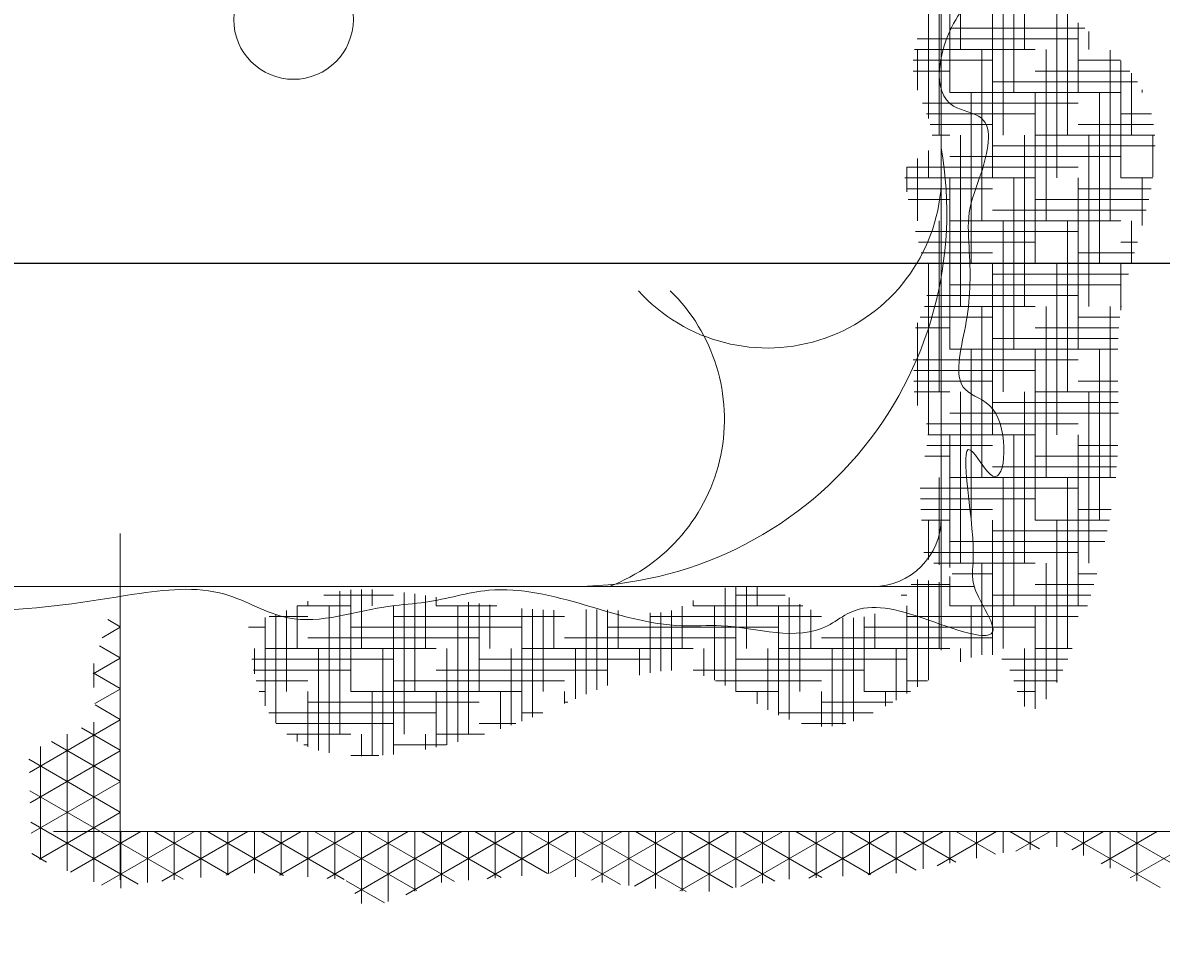
# Model space of a CAD drawing. Units: inches. Extents: x 3731 to 4318, y 1310 to 2388.
# Tile 52 of 57: x 4157 to 4212, y 2229 to 2274. Entities that reach past the tile are written whole.
import ezdxf

# ---------------------------------------------------------------- set-up
doc = ezdxf.new("R2010")
doc.units = ezdxf.units.IN
doc.layers.add('A-ANNO-DIMS', color=2, linetype='Continuous', lineweight=18)
doc.layers.add('A-FURN', color=8, linetype='Continuous', lineweight=13)
doc.styles.get("Standard").update_dxf_attribs({"font": 'arial.ttf'})
doc.dimstyles.get("Standard").update_dxf_attribs({"dimtxt": 0.18, "dimasz": 0.18, "dimexe": 0.18, "dimexo": 0.0625, "dimgap": 0.09, "dimtad": 0, "dimtih": 1, "dimtoh": 1, "dimdec": 4, "dimzin": 0, "dimdsep": 46, "dimtxsty": 'Standard', "dimcen": 0.09, "dimadec": 0, "dimazin": 0, "dimtfac": 1, "dimtdec": 4, "dimtofl": 0, "dimtmove": 0, "dimatfit": 3, "dimfxl": 1, "dimtolj": 1, "dimtzin": 0, "dimarcsym": 0})

# ---------------------------------------------------------------- blocks, each defined once
blk = doc.blocks.new('A$C200C7901')
for p, q in [((2, 0.2957), (2, 1.2957)), ((2.0224, 0.9977), (2.0224, 1.1977)), ((2.0224, 0.9977), (2.0224, 1.1977)), ((1.9974, 0.5977), (1.9974, 0.7977)), ((1.9974, 0.5977), (1.9974, 0.7977)), ((2.0724, 0.5977), (2.0724, 0.7977)), ((2.0724, 0.5977), (2.0724, 0.7977)), ((2.1474, 0.5977), (2.1474, 0.7977)), ((2.1474, 0.5977), (2.1474, 0.7977)), ((1.9849, 0.5477), (1.9849, 0.7477)), ((1.9849, 0.5477), (1.9849, 0.7477)), ((2.0599, 0.5477), (2.0599, 0.7477)), ((2.0599, 0.5477), (2.0599, 0.7477)), ((2.1349, 0.5477), (2.1349, 0.7477)), ((2.1349, 0.5477), (2.1349, 0.7477)), ((1.0407, 0.0275), (1.0407, 0.4323)), ((0.4061, 0.3703), (2.0386, 0.3703)), ((2.4073, 0.0839), (0.9625, 0.0839))]:
    blk.add_line(p, q)
at = {"linetype": 'ByBlock'}
for p, q in [((2.0099, 0.9477), (2.0099, 1.1477)), ((2.0099, 0.9477), (2.0099, 1.1477)), ((2.0849, 0.9477), (2.0849, 1.1477)), ((2.0849, 0.9477), (2.0849, 1.1477)), ((1.9974, 0.8977), (1.9974, 1.0977)), ((1.9974, 0.8977), (1.9974, 1.0977)), ((2.0724, 0.8977), (2.0724, 1.0977)), ((2.0724, 0.8977), (2.0724, 1.0977)), ((2.0974, 0.9977), (2.0974, 1.0909)), ((2.0974, 0.9977), (2.0974, 1.0909)), ((1.9849, 0.9171), (1.9849, 1.0477)), ((1.9849, 0.9171), (1.9849, 1.0477)), ((2.0599, 0.8477), (2.0599, 1.0477)), ((2.0599, 0.8477), (2.0599, 1.0477)), ((2.1349, 0.8477), (2.1349, 1.0477)), ((2.1349, 0.8477), (2.1349, 1.0477)), ((2.1474, 0.8977), (2.1474, 1.0391)), ((2.1474, 0.8977), (2.1474, 1.0391)), ((2.1599, 0.9477), (2.1599, 1.029)), ((2.1599, 0.9477), (2.1599, 1.029)), ((2.0099, 1.0227), (2.1678, 1.0227)), ((2.0099, 1.0227), (2.1678, 1.0227)), ((2.1724, 0.9977), (2.1724, 1.0189)), ((2.1724, 0.9977), (2.1724, 1.0189)), ((1.9718, 1.0102), (2.1599, 1.0102)), ((1.9718, 1.0102), (2.1599, 1.0102)), ((1.9671, 0.9852), (2.0599, 0.9852)), ((1.9671, 0.9852), (2.0599, 0.9852)), ((1.9688, 0.9977), (2.1099, 0.9977)), ((1.9688, 0.9977), (2.1099, 0.9977)), ((1.9724, 0.9504), (1.9724, 0.9977)), ((1.9724, 0.9504), (1.9724, 0.9977)), ((2.0474, 0.7977), (2.0474, 0.9977)), ((2.0474, 0.7977), (2.0474, 0.9977)), ((2.1224, 0.7977), (2.1224, 0.9977)), ((2.1224, 0.7977), (2.1224, 0.9977)), ((2.1599, 0.9852), (2.2095, 0.9852)), ((2.1599, 0.9852), (2.2095, 0.9852)), ((2.1974, 0.7977), (2.1974, 0.9972)), ((2.1974, 0.7977), (2.1974, 0.9972)), ((2.2099, 0.8477), (2.2099, 0.9848)), ((2.2099, 0.8477), (2.2099, 0.9848)), ((1.9672, 0.9727), (2.0099, 0.9727)), ((1.9672, 0.9727), (2.0099, 0.9727)), ((2.1099, 0.9727), (2.2204, 0.9727)), ((2.1099, 0.9727), (2.2204, 0.9727)), ((2.0599, 0.9602), (2.2294, 0.9602)), ((2.0599, 0.9602), (2.2294, 0.9602)), ((2.2224, 0.8977), (2.2224, 0.9702)), ((2.2224, 0.8977), (2.2224, 0.9702)), ((2.0099, 0.9477), (2.2099, 0.9477)), ((2.0099, 0.9477), (2.2099, 0.9477)), ((2.0349, 0.7477), (2.0349, 0.9477)), ((2.0349, 0.7477), (2.0349, 0.9477)), ((2.1099, 0.7477), (2.1099, 0.9477)), ((2.1099, 0.7477), (2.1099, 0.9477)), ((2.1849, 0.7477), (2.1849, 0.9477)), ((2.1849, 0.7477), (2.1849, 0.9477)), ((2.2349, 0.9477), (2.2349, 0.9506)), ((2.2349, 0.9477), (2.2349, 0.9506)), ((1.9781, 0.9352), (2.1599, 0.9352)), ((1.9781, 0.9352), (2.1599, 0.9352)), ((1.9829, 0.9227), (2.1099, 0.9227)), ((1.9829, 0.9227), (2.1099, 0.9227)), ((2.2099, 0.9227), (2.2455, 0.9227)), ((2.2099, 0.9227), (2.2455, 0.9227)), ((1.9871, 0.9102), (2.0599, 0.9102)), ((1.9871, 0.9102), (2.0599, 0.9102)), ((2.1599, 0.9102), (2.2481, 0.9102)), ((2.1599, 0.9102), (2.2481, 0.9102)), ((1.9894, 0.8977), (2.0099, 0.8977)), ((1.9894, 0.8977), (2.0099, 0.8977)), ((2.0224, 0.6977), (2.0224, 0.8977)), ((2.0224, 0.6977), (2.0224, 0.8977)), ((2.0974, 0.6977), (2.0974, 0.8977)), ((2.0974, 0.6977), (2.0974, 0.8977)), ((2.1099, 0.8977), (2.2496, 0.8977)), ((2.1099, 0.8977), (2.2496, 0.8977)), ((2.1724, 0.6977), (2.1724, 0.8977)), ((2.1724, 0.6977), (2.1724, 0.8977)), ((2.2474, 0.8489), (2.2474, 0.8977)), ((2.2474, 0.8489), (2.2474, 0.8977)), ((1.9849, 0.8477), (1.9849, 0.88)), ((1.9849, 0.8477), (1.9849, 0.88)), ((2.0599, 0.8852), (2.2501, 0.8852)), ((2.0599, 0.8852), (2.2501, 0.8852)), ((1.9724, 0.7977), (1.9724, 0.8703)), ((1.9724, 0.7977), (1.9724, 0.8703)), ((2.0099, 0.8727), (2.2099, 0.8727)), ((2.0099, 0.8727), (2.2099, 0.8727)), ((1.9599, 0.8317), (1.9599, 0.8604)), ((1.9599, 0.8317), (1.9599, 0.8604)), ((1.9599, 0.8602), (2.1599, 0.8602)), ((1.9599, 0.8602), (2.1599, 0.8602)), ((1.9574, 0.8477), (2.1099, 0.8477)), ((1.9574, 0.8477), (2.1099, 0.8477)), ((2.0099, 0.6477), (2.0099, 0.8477)), ((2.0099, 0.6477), (2.0099, 0.8477)), ((2.0849, 0.6477), (2.0849, 0.8477)), ((2.0849, 0.6477), (2.0849, 0.8477)), ((2.1599, 0.6477), (2.1599, 0.8477)), ((2.1599, 0.6477), (2.1599, 0.8477)), ((2.2099, 0.8477), (2.2472, 0.8477)), ((2.2099, 0.8477), (2.2472, 0.8477)), ((2.2349, 0.7923), (2.2349, 0.8477)), ((2.2349, 0.7923), (2.2349, 0.8477)), ((1.9593, 0.8352), (2.0599, 0.8352)), ((1.9593, 0.8352), (2.0599, 0.8352)), ((2.1599, 0.8352), (2.2451, 0.8352)), ((2.1599, 0.8352), (2.2451, 0.8352)), ((1.9615, 0.8227), (2.0099, 0.8227)), ((1.9615, 0.8227), (2.0099, 0.8227)), ((2.1099, 0.8227), (2.2425, 0.8227)), ((2.1099, 0.8227), (2.2425, 0.8227)), ((2.0599, 0.8102), (2.2396, 0.8102)), ((2.0599, 0.8102), (2.2396, 0.8102)), ((1.9699, 0.7852), (2.1599, 0.7852)), ((1.9699, 0.7852), (2.1599, 0.7852)), ((2.0099, 0.7977), (2.2099, 0.7977)), ((2.0099, 0.7977), (2.2099, 0.7977)), ((2.2224, 0.7483), (2.2224, 0.7977)), ((2.2224, 0.7483), (2.2224, 0.7977)), ((1.9734, 0.7727), (2.1099, 0.7727)), ((1.9734, 0.7727), (2.1099, 0.7727)), ((2.2099, 0.7727), (2.2294, 0.7727)), ((2.2099, 0.7727), (2.2294, 0.7727)), ((1.9767, 0.7602), (2.0599, 0.7602)), ((1.9767, 0.7602), (2.0599, 0.7602)), ((2.1599, 0.7602), (2.2258, 0.7602)), ((2.1599, 0.7602), (2.2258, 0.7602)), ((1.9797, 0.7477), (2.0099, 0.7477)), ((1.9797, 0.7477), (2.0099, 0.7477)), ((2.1099, 0.7477), (2.2222, 0.7477)), ((2.1099, 0.7477), (2.2222, 0.7477)), ((2.2099, 0.6933), (2.2099, 0.7477)), ((2.2099, 0.6933), (2.2099, 0.7477)), ((2.0599, 0.7352), (2.2188, 0.7352)), ((2.0599, 0.7352), (2.2188, 0.7352)), ((2.0099, 0.7227), (2.2099, 0.7227)), ((2.0099, 0.7227), (2.2099, 0.7227)), ((1.9831, 0.7102), (2.1599, 0.7102)), ((1.9831, 0.7102), (2.1599, 0.7102)), ((1.9804, 0.6977), (2.1099, 0.6977)), ((1.9804, 0.6977), (2.1099, 0.6977)), ((2.0474, 0.4977), (2.0474, 0.6977)), ((2.0474, 0.4977), (2.0474, 0.6977)), ((2.1224, 0.4977), (2.1224, 0.6977)), ((2.1224, 0.4977), (2.1224, 0.6977)), ((2.1974, 0.4977), (2.1974, 0.6977)), ((2.1974, 0.4977), (2.1974, 0.6977)), ((2.2099, 0.6977), (2.2106, 0.6977)), ((2.2099, 0.6977), (2.2106, 0.6977)), ((1.9724, 0.5818), (1.9724, 0.6786)), ((1.9724, 0.5818), (1.9724, 0.6786)), ((1.9753, 0.6852), (2.0599, 0.6852)), ((1.9753, 0.6852), (2.0599, 0.6852)), ((2.1599, 0.6852), (2.2088, 0.6852)), ((2.1599, 0.6852), (2.2088, 0.6852)), ((1.97, 0.6727), (2.0099, 0.6727)), ((1.97, 0.6727), (2.0099, 0.6727)), ((2.1099, 0.6727), (2.2075, 0.6727)), ((2.1099, 0.6727), (2.2075, 0.6727)), ((2.0599, 0.6602), (2.2067, 0.6602)), ((2.0599, 0.6602), (2.2067, 0.6602)), ((2.0099, 0.6477), (2.2062, 0.6477)), ((2.0099, 0.6477), (2.2062, 0.6477)), ((2.0349, 0.4477), (2.0349, 0.6477)), ((2.0349, 0.4477), (2.0349, 0.6477)), ((2.1099, 0.4477), (2.1099, 0.6477)), ((2.1099, 0.4477), (2.1099, 0.6477)), ((2.1849, 0.4477), (2.1849, 0.6477)), ((2.1849, 0.4477), (2.1849, 0.6477)), ((1.9673, 0.6352), (2.1599, 0.6352)), ((1.9673, 0.6352), (2.1599, 0.6352)), ((1.9678, 0.6227), (2.1099, 0.6227)), ((1.9678, 0.6227), (2.1099, 0.6227)), ((1.9679, 0.6102), (2.0599, 0.6102)), ((1.9679, 0.6102), (2.0599, 0.6102)), ((2.1599, 0.6102), (2.2064, 0.6102)), ((2.1599, 0.6102), (2.2064, 0.6102)), ((1.9685, 0.5977), (2.0099, 0.5977)), ((1.9685, 0.5977), (2.0099, 0.5977)), ((2.0224, 0.3977), (2.0224, 0.5977)), ((2.0224, 0.3977), (2.0224, 0.5977)), ((2.0974, 0.3977), (2.0974, 0.5977)), ((2.0974, 0.3977), (2.0974, 0.5977)), ((2.1099, 0.5977), (2.2066, 0.5977)), ((2.1099, 0.5977), (2.2066, 0.5977)), ((2.1724, 0.3977), (2.1724, 0.5977)), ((2.1724, 0.3977), (2.1724, 0.5977)), ((2.0099, 0.5727), (2.207, 0.5727)), ((2.0099, 0.5727), (2.207, 0.5727)), ((2.0599, 0.5852), (2.2069, 0.5852)), ((2.0599, 0.5852), (2.2069, 0.5852)), ((1.9827, 0.5602), (2.1599, 0.5602)), ((1.9827, 0.5602), (2.1599, 0.5602)), ((1.9842, 0.5477), (2.1099, 0.5477)), ((1.9842, 0.5477), (2.1099, 0.5477)), ((2.0099, 0.3923), (2.0099, 0.5477)), ((2.0099, 0.3923), (2.0099, 0.5477)), ((2.0849, 0.3477), (2.0849, 0.5477)), ((2.0849, 0.3477), (2.0849, 0.5477)), ((2.1599, 0.3477), (2.1599, 0.5477)), ((2.1599, 0.3477), (2.1599, 0.5477)), ((1.9831, 0.5352), (2.0599, 0.5352)), ((1.9831, 0.5352), (2.0599, 0.5352)), ((2.1599, 0.5352), (2.2065, 0.5352)), ((2.1599, 0.5352), (2.2065, 0.5352)), ((1.9807, 0.5227), (2.0099, 0.5227)), ((1.9807, 0.5227), (2.0099, 0.5227)), ((2.1099, 0.5227), (2.2058, 0.5227)), ((2.1099, 0.5227), (2.2058, 0.5227)), ((2.0599, 0.5102), (2.2049, 0.5102)), ((2.0599, 0.5102), (2.2049, 0.5102)), ((1.9974, 0.3957), (1.9974, 0.4977)), ((1.9974, 0.3957), (1.9974, 0.4977)), ((2.0099, 0.4977), (2.2038, 0.4977)), ((2.0099, 0.4977), (2.2038, 0.4977)), ((2.0724, 0.2977), (2.0724, 0.4977)), ((2.0724, 0.2977), (2.0724, 0.4977)), ((2.1474, 0.2977), (2.1474, 0.4977)), ((2.1474, 0.2977), (2.1474, 0.4977)), ((1.9755, 0.4852), (2.1599, 0.4852)), ((1.9755, 0.4852), (2.1599, 0.4852)), ((1.9757, 0.4727), (2.1099, 0.4727)), ((1.9757, 0.4727), (2.1099, 0.4727)), ((1.9762, 0.4602), (2.0599, 0.4602)), ((1.9762, 0.4602), (2.0599, 0.4602)), ((2.1599, 0.4602), (2.1987, 0.4602)), ((2.1599, 0.4602), (2.1987, 0.4602)), ((1.9768, 0.4477), (2.0099, 0.4477)), ((1.9768, 0.4477), (2.0099, 0.4477)), ((1.9849, 0.402), (1.9849, 0.4477)), ((1.9849, 0.402), (1.9849, 0.4477)), ((2.0599, 0.2903), (2.0599, 0.4477)), ((2.0599, 0.2903), (2.0599, 0.4477)), ((2.1099, 0.4477), (2.1965, 0.4477)), ((2.1099, 0.4477), (2.1965, 0.4477)), ((2.1349, 0.2582), (2.1349, 0.4477)), ((2.1349, 0.2582), (2.1349, 0.4477)), ((2.0599, 0.4352), (2.194, 0.4352)), ((2.0599, 0.4352), (2.194, 0.4352)), ((2.0099, 0.4227), (2.1913, 0.4227)), ((2.0099, 0.4227), (2.1913, 0.4227)), ((1.9797, 0.4102), (2.1599, 0.4102)), ((1.9797, 0.4102), (2.1599, 0.4102)), ((1.9915, 0.3977), (2.1099, 0.3977)), ((1.9915, 0.3977), (2.1099, 0.3977)), ((2.0474, 0.2905), (2.0474, 0.3977)), ((2.0474, 0.2905), (2.0474, 0.3977)), ((2.1224, 0.2385), (2.1224, 0.3977)), ((2.1224, 0.2385), (2.1224, 0.3977)), ((1.9648, 0.3727), (2.0099, 0.3727)), ((1.9648, 0.3727), (2.0099, 0.3727)), ((1.9724, 0.253), (1.9724, 0.3785)), ((1.9724, 0.253), (1.9724, 0.3785)), ((1.9849, 0.2609), (1.9849, 0.3774)), ((1.9849, 0.2609), (1.9849, 0.3774)), ((1.9974, 0.2977), (1.9974, 0.3753)), ((1.9974, 0.2977), (1.9974, 0.3753)), ((2.0099, 0.3477), (2.0099, 0.382)), ((2.0099, 0.3477), (2.0099, 0.382)), ((2.0127, 0.3852), (2.0599, 0.3852)), ((2.0127, 0.3852), (2.0599, 0.3852)), ((2.1099, 0.3727), (2.1784, 0.3727)), ((2.1099, 0.3727), (2.1784, 0.3727)), ((2.1599, 0.3852), (2.1819, 0.3852)), ((2.1599, 0.3852), (2.1819, 0.3852)), ((1.2785, 0.3602), (1.3599, 0.3602)), ((1.2785, 0.3602), (1.3599, 0.3602)), ((1.2974, 0.1977), (1.2974, 0.3647)), ((1.2974, 0.1977), (1.2974, 0.3647)), ((1.3099, 0.2477), (1.3099, 0.3663)), ((1.3099, 0.2477), (1.3099, 0.3663)), ((1.3224, 0.2977), (1.3224, 0.3669)), ((1.3224, 0.2977), (1.3224, 0.3669)), ((1.3349, 0.3477), (1.3349, 0.3668)), ((1.3349, 0.3477), (1.3349, 0.3668)), ((1.3724, 0.1977), (1.3724, 0.3634)), ((1.3724, 0.1977), (1.3724, 0.3634)), ((1.3849, 0.2477), (1.3849, 0.3616)), ((1.3849, 0.2477), (1.3849, 0.3616)), ((1.3974, 0.2977), (1.3974, 0.3597)), ((1.3974, 0.2977), (1.3974, 0.3597)), ((1.7474, 0.2546), (1.7474, 0.3689)), ((1.7474, 0.2546), (1.7474, 0.3689)), ((1.7599, 0.2477), (1.7599, 0.3703)), ((1.7599, 0.2477), (1.7599, 0.3703)), ((1.7599, 0.3602), (1.8177, 0.3602)), ((1.7599, 0.3602), (1.8177, 0.3602)), ((1.7724, 0.2977), (1.7724, 0.3703)), ((1.7724, 0.2977), (1.7724, 0.3703)), ((1.7849, 0.3477), (1.7849, 0.3703)), ((1.7849, 0.3477), (1.7849, 0.3703)), ((1.9532, 0.3602), (1.9599, 0.3602)), ((1.9532, 0.3602), (1.9599, 0.3602)), ((2.0599, 0.3602), (2.1747, 0.3602)), ((2.0599, 0.3602), (2.1747, 0.3602)), ((1.2474, 0.2977), (1.2474, 0.3476)), ((1.2474, 0.2977), (1.2474, 0.3476)), ((1.2475, 0.3477), (1.3099, 0.3477)), ((1.2475, 0.3477), (1.3099, 0.3477)), ((1.2599, 0.3477), (1.2599, 0.3531)), ((1.2599, 0.3477), (1.2599, 0.3531)), ((1.2849, 0.1758), (1.2849, 0.3477)), ((1.2849, 0.1758), (1.2849, 0.3477)), ((1.3599, 0.1741), (1.3599, 0.3477)), ((1.3599, 0.1741), (1.3599, 0.3477)), ((1.4099, 0.3477), (1.4099, 0.3578)), ((1.4099, 0.3477), (1.4099, 0.3578)), ((1.4099, 0.3477), (1.4806, 0.3477)), ((1.4099, 0.3477), (1.4806, 0.3477)), ((1.4349, 0.1886), (1.4349, 0.3477)), ((1.4349, 0.1886), (1.4349, 0.3477)), ((1.4474, 0.1977), (1.4474, 0.3521)), ((1.4474, 0.1977), (1.4474, 0.3521)), ((1.4599, 0.2477), (1.4599, 0.3504)), ((1.4599, 0.2477), (1.4599, 0.3504)), ((1.4724, 0.2977), (1.4724, 0.3487)), ((1.4724, 0.2977), (1.4724, 0.3487)), ((1.6974, 0.2977), (1.6974, 0.3472)), ((1.6974, 0.2977), (1.6974, 0.3472)), ((1.7099, 0.3477), (1.7099, 0.3539)), ((1.7099, 0.3477), (1.7099, 0.3539)), ((1.7099, 0.3477), (1.8383, 0.3477)), ((1.7099, 0.3477), (1.8383, 0.3477)), ((1.7349, 0.2607), (1.7349, 0.3477)), ((1.7349, 0.2607), (1.7349, 0.3477)), ((1.8099, 0.2201), (1.8099, 0.3477)), ((1.8099, 0.2201), (1.8099, 0.3477)), ((1.8224, 0.2148), (1.8224, 0.3575)), ((1.8224, 0.2148), (1.8224, 0.3575)), ((1.8349, 0.2477), (1.8349, 0.3497)), ((1.8349, 0.2477), (1.8349, 0.3497)), ((1.9599, 0.2452), (1.9599, 0.3477)), ((1.9599, 0.2452), (1.9599, 0.3477)), ((2.0099, 0.3477), (2.1708, 0.3477)), ((2.0099, 0.3477), (2.1708, 0.3477)), ((2.0349, 0.2874), (2.0349, 0.3477)), ((2.0349, 0.2874), (2.0349, 0.3477)), ((2.1099, 0.2274), (2.1099, 0.3477)), ((2.1099, 0.2274), (2.1099, 0.3477)), ((1.2099, 0.2308), (1.2099, 0.334)), ((1.2099, 0.2308), (1.2099, 0.334)), ((1.2148, 0.3352), (1.2599, 0.3352)), ((1.2148, 0.3352), (1.2599, 0.3352)), ((1.2224, 0.2106), (1.2224, 0.3375)), ((1.2224, 0.2106), (1.2224, 0.3375)), ((1.2349, 0.2477), (1.2349, 0.3422)), ((1.2349, 0.2477), (1.2349, 0.3422)), ((1.3599, 0.3352), (1.5599, 0.3352)), ((1.3599, 0.3352), (1.5599, 0.3352)), ((1.5099, 0.2129), (1.5099, 0.3447)), ((1.5099, 0.2129), (1.5099, 0.3447)), ((1.5224, 0.2177), (1.5224, 0.3438)), ((1.5224, 0.2177), (1.5224, 0.3438)), ((1.5349, 0.2477), (1.5349, 0.3431)), ((1.5349, 0.2477), (1.5349, 0.3431)), ((1.5474, 0.2977), (1.5474, 0.3428)), ((1.5474, 0.2977), (1.5474, 0.3428)), ((1.5849, 0.2443), (1.5849, 0.3434)), ((1.5849, 0.2443), (1.5849, 0.3434)), ((1.5974, 0.2496), (1.5974, 0.3435)), ((1.5974, 0.2496), (1.5974, 0.3435)), ((1.6099, 0.2546), (1.6099, 0.3432)), ((1.6099, 0.2546), (1.6099, 0.3432)), ((1.6224, 0.2977), (1.6224, 0.3424)), ((1.6224, 0.2977), (1.6224, 0.3424)), ((1.6599, 0.2695), (1.6599, 0.3394)), ((1.6599, 0.2695), (1.6599, 0.3394)), ((1.6599, 0.3352), (1.8599, 0.3352)), ((1.6599, 0.3352), (1.8599, 0.3352)), ((1.6724, 0.2713), (1.6724, 0.3398)), ((1.6724, 0.2713), (1.6724, 0.3398)), ((1.6849, 0.272), (1.6849, 0.3422)), ((1.6849, 0.272), (1.6849, 0.3422)), ((1.8474, 0.2977), (1.8474, 0.3432)), ((1.8474, 0.2977), (1.8474, 0.3432)), ((1.8849, 0.2093), (1.8849, 0.3337)), ((1.8849, 0.2093), (1.8849, 0.3337)), ((1.8974, 0.2129), (1.8974, 0.3335)), ((1.8974, 0.2129), (1.8974, 0.3335)), ((1.9099, 0.2477), (1.9099, 0.3349)), ((1.9099, 0.2477), (1.9099, 0.3349)), ((1.9224, 0.2977), (1.9224, 0.3385)), ((1.9224, 0.2977), (1.9224, 0.3385)), ((1.9599, 0.3352), (2.1599, 0.3352)), ((1.9599, 0.3352), (2.1599, 0.3352)), ((1.0194, 0.3103), (1.0407, 0.3227)), ((1.0194, 0.3103), (1.0407, 0.3227)), ((1.0261, 0.3316), (1.0407, 0.3232)), ((1.0261, 0.3316), (1.0407, 0.3232)), ((1.1904, 0.3227), (1.2099, 0.3227)), ((1.1904, 0.3227), (1.2099, 0.3227)), ((1.3099, 0.3227), (1.5099, 0.3227)), ((1.3099, 0.3227), (1.5099, 0.3227)), ((1.6099, 0.3227), (1.8099, 0.3227)), ((1.6099, 0.3227), (1.8099, 0.3227)), ((1.9099, 0.3227), (2.1099, 0.3227)), ((1.9099, 0.3227), (2.1099, 0.3227)), ((1.2599, 0.3102), (1.4599, 0.3102)), ((1.2599, 0.3102), (1.4599, 0.3102)), ((1.5599, 0.3102), (1.7599, 0.3102)), ((1.5599, 0.3102), (1.7599, 0.3102)), ((1.8599, 0.3102), (2.0599, 0.3102)), ((1.8599, 0.3102), (2.0599, 0.3102)), ((1.0164, 0.3011), (1.0407, 0.2871)), ((1.0164, 0.3011), (1.0407, 0.2871)), ((1.1974, 0.2683), (1.1974, 0.2977)), ((1.1974, 0.2683), (1.1974, 0.2977)), ((1.2099, 0.2977), (1.4099, 0.2977)), ((1.2099, 0.2977), (1.4099, 0.2977)), ((1.2724, 0.1788), (1.2724, 0.2977)), ((1.2724, 0.1788), (1.2724, 0.2977)), ((1.3474, 0.173), (1.3474, 0.2977)), ((1.3474, 0.173), (1.3474, 0.2977)), ((1.4224, 0.1854), (1.4224, 0.2977)), ((1.4224, 0.1854), (1.4224, 0.2977)), ((1.4974, 0.2083), (1.4974, 0.2977)), ((1.4974, 0.2083), (1.4974, 0.2977)), ((1.5099, 0.2977), (1.7099, 0.2977)), ((1.5099, 0.2977), (1.7099, 0.2977)), ((1.5724, 0.2389), (1.5724, 0.2977)), ((1.5724, 0.2389), (1.5724, 0.2977)), ((1.6474, 0.2668), (1.6474, 0.2977)), ((1.6474, 0.2668), (1.6474, 0.2977)), ((1.7224, 0.2658), (1.7224, 0.2977)), ((1.7224, 0.2658), (1.7224, 0.2977)), ((1.7974, 0.2263), (1.7974, 0.2977)), ((1.7974, 0.2263), (1.7974, 0.2977)), ((1.8099, 0.2977), (2.0099, 0.2977)), ((1.8099, 0.2977), (2.0099, 0.2977)), ((1.8724, 0.2072), (1.8724, 0.2977)), ((1.8724, 0.2072), (1.8724, 0.2977)), ((1.9474, 0.2376), (1.9474, 0.2977)), ((1.9474, 0.2376), (1.9474, 0.2977)), ((2.0224, 0.2822), (2.0224, 0.2977)), ((2.0224, 0.2822), (2.0224, 0.2977)), ((2.0974, 0.2299), (2.0974, 0.2977)), ((2.0974, 0.2299), (2.0974, 0.2977)), ((2.1099, 0.2977), (2.153, 0.2977)), ((2.1099, 0.2977), (2.153, 0.2977)), ((1.0089, 0.2682), (1.0407, 0.2866)), ((1.0089, 0.2682), (1.0407, 0.2866)), ((1.0099, 0.2521), (1.0099, 0.2804)), ((1.0099, 0.2521), (1.0099, 0.2804)), ((1.1943, 0.2852), (1.3599, 0.2852)), ((1.1943, 0.2852), (1.3599, 0.2852)), ((1.4599, 0.2852), (1.6599, 0.2852)), ((1.4599, 0.2852), (1.6599, 0.2852)), ((1.7599, 0.2852), (1.9599, 0.2852)), ((1.7599, 0.2852), (1.9599, 0.2852)), ((2.0708, 0.2852), (2.1478, 0.2852)), ((2.0708, 0.2852), (2.1478, 0.2852)), ((1.0088, 0.2694), (1.0407, 0.251)), ((1.0088, 0.2694), (1.0407, 0.251)), ((1.1965, 0.2727), (1.3099, 0.2727)), ((1.1965, 0.2727), (1.3099, 0.2727)), ((1.4099, 0.2727), (1.6099, 0.2727)), ((1.4099, 0.2727), (1.6099, 0.2727)), ((1.7099, 0.2727), (1.9099, 0.2727)), ((1.7099, 0.2727), (1.9099, 0.2727)), ((2.08, 0.2727), (2.1422, 0.2727)), ((2.08, 0.2727), (2.1422, 0.2727)), ((1.1994, 0.2602), (1.2599, 0.2602)), ((1.1994, 0.2602), (1.2599, 0.2602)), ((1.3599, 0.2602), (1.5599, 0.2602)), ((1.3599, 0.2602), (1.5599, 0.2602)), ((1.7361, 0.2602), (1.8599, 0.2602)), ((1.7361, 0.2602), (1.8599, 0.2602)), ((1.9599, 0.2602), (1.9838, 0.2602)), ((1.9599, 0.2602), (1.9838, 0.2602)), ((2.0848, 0.2602), (2.1359, 0.2602)), ((2.0848, 0.2602), (2.1359, 0.2602)), ((1.0111, 0.2334), (1.0407, 0.2505)), ((1.0111, 0.2334), (1.0407, 0.2505)), ((1.2031, 0.2477), (1.2099, 0.2477)), ((1.2031, 0.2477), (1.2099, 0.2477)), ((1.2599, 0.1831), (1.2599, 0.2477)), ((1.2599, 0.1831), (1.2599, 0.2477)), ((1.3099, 0.2477), (1.5099, 0.2477)), ((1.3099, 0.2477), (1.5099, 0.2477)), ((1.3349, 0.1723), (1.3349, 0.2477)), ((1.3349, 0.1723), (1.3349, 0.2477)), ((1.4099, 0.1825), (1.4099, 0.2477)), ((1.4099, 0.1825), (1.4099, 0.2477)), ((1.4849, 0.2039), (1.4849, 0.2477)), ((1.4849, 0.2039), (1.4849, 0.2477)), ((1.5599, 0.2335), (1.5599, 0.2477)), ((1.5599, 0.2335), (1.5599, 0.2477)), ((1.7599, 0.2477), (1.8099, 0.2477)), ((1.7599, 0.2477), (1.8099, 0.2477)), ((1.7849, 0.2332), (1.7849, 0.2477)), ((1.7849, 0.2332), (1.7849, 0.2477)), ((1.8599, 0.2068), (1.8599, 0.2477)), ((1.8599, 0.2068), (1.8599, 0.2477)), ((1.9099, 0.2477), (1.9639, 0.2477)), ((1.9099, 0.2477), (1.9639, 0.2477)), ((1.9349, 0.2304), (1.9349, 0.2477)), ((1.9349, 0.2304), (1.9349, 0.2477)), ((2.0888, 0.2477), (2.1099, 0.2477)), ((2.0888, 0.2477), (2.1099, 0.2477)), ((1.0112, 0.232), (1.0407, 0.215)), ((1.0112, 0.232), (1.0407, 0.215)), ((1.2599, 0.2352), (1.4599, 0.2352)), ((1.2599, 0.2352), (1.4599, 0.2352)), ((1.5599, 0.2352), (1.5638, 0.2352)), ((1.5599, 0.2352), (1.5638, 0.2352)), ((1.8599, 0.2352), (1.9433, 0.2352)), ((1.8599, 0.2352), (1.9433, 0.2352)), ((0.9344, 0.153), (1.0407, 0.2144)), ((0.9344, 0.153), (1.0407, 0.2144)), ((1.2142, 0.2227), (1.4099, 0.2227)), ((1.2142, 0.2227), (1.4099, 0.2227)), ((1.5099, 0.2227), (1.5346, 0.2227)), ((1.5099, 0.2227), (1.5346, 0.2227)), ((1.8099, 0.2227), (1.9203, 0.2227)), ((1.8099, 0.2227), (1.9203, 0.2227)), ((0.9953, 0.2051), (1.0407, 0.1789)), ((0.9953, 0.2051), (1.0407, 0.1789)), ((1.0099, 0.0251), (1.0099, 0.2117)), ((1.0099, 0.0251), (1.0099, 0.2117)), ((1.2227, 0.2102), (1.3599, 0.2102)), ((1.2227, 0.2102), (1.3599, 0.2102)), ((1.4599, 0.2102), (1.5027, 0.2102)), ((1.4599, 0.2102), (1.5027, 0.2102)), ((1.8368, 0.2102), (1.8884, 0.2102)), ((1.8368, 0.2102), (1.8884, 0.2102)), ((0.9602, 0.1893), (1.0407, 0.1428)), ((0.9602, 0.1893), (1.0407, 0.1428)), ((0.9787, 0.0381), (0.9787, 0.1976)), ((0.9787, 0.0381), (0.9787, 0.1976)), ((1.2351, 0.1977), (1.3099, 0.1977)), ((1.2351, 0.1977), (1.3099, 0.1977)), ((1.2474, 0.1892), (1.2474, 0.1977)), ((1.2474, 0.1892), (1.2474, 0.1977)), ((1.3224, 0.1722), (1.3224, 0.1977)), ((1.3224, 0.1722), (1.3224, 0.1977)), ((1.3974, 0.1799), (1.3974, 0.1977)), ((1.3974, 0.1799), (1.3974, 0.1977)), ((1.4099, 0.1977), (1.4662, 0.1977)), ((1.4099, 0.1977), (1.4662, 0.1977)), ((0.9355, 0.1176), (1.0407, 0.1783)), ((0.9355, 0.1176), (1.0407, 0.1783)), ((0.9474, 0.0512), (0.9474, 0.1835)), ((0.9474, 0.0512), (0.9474, 0.1835)), ((1.2552, 0.1852), (1.2599, 0.1852)), ((1.2552, 0.1852), (1.2599, 0.1852)), ((1.3599, 0.1852), (1.4215, 0.1852)), ((1.3599, 0.1852), (1.4215, 0.1852)), ((0.9339, 0.1684), (1.0407, 0.1067)), ((0.9339, 0.1684), (1.0407, 0.1067)), ((1.3099, 0.1727), (1.3428, 0.1727)), ((1.3099, 0.1727), (1.3428, 0.1727)), ((0.9366, 0.0822), (1.0407, 0.1422)), ((0.9366, 0.0822), (1.0407, 0.1422)), ((2.2208, 0.0297), (2.4078, 0.1377)), ((2.2208, 0.0297), (2.4078, 0.1377)), ((0.935, 0.1316), (1.114, 0.0283)), ((0.935, 0.1316), (1.114, 0.0283)), ((0.9362, 0.0948), (1.0616, 0.0225)), ((0.9362, 0.0948), (1.0616, 0.0225)), ((0.9463, 0.0516), (1.0407, 0.1061)), ((0.9463, 0.0516), (1.0407, 0.1061)), ((0.9826, 0.0365), (1.0647, 0.0839)), ((0.9826, 0.0365), (1.0647, 0.0839)), ((1.0189, 0.0214), (1.1272, 0.0839)), ((1.0189, 0.0214), (1.1272, 0.0839)), ((1.0412, 0.0179), (1.0412, 0.0839)), ((1.0412, 0.0179), (1.0412, 0.0839)), ((1.0724, 0.0243), (1.0724, 0.0839)), ((1.0724, 0.0243), (1.0724, 0.0839)), ((1.0801, 0.0839), (1.1675, 0.0335)), ((1.0801, 0.0839), (1.1675, 0.0335)), ((1.0891, 0.0259), (1.1897, 0.0839)), ((1.0891, 0.0259), (1.1897, 0.0839)), ((1.1037, 0.0273), (1.1037, 0.0839)), ((1.1037, 0.0273), (1.1037, 0.0839)), ((1.1349, 0.0303), (1.1349, 0.0839)), ((1.1349, 0.0303), (1.1349, 0.0839)), ((1.1426, 0.0839), (1.2313, 0.0327)), ((1.1426, 0.0839), (1.2313, 0.0327)), ((1.1642, 0.0331), (1.2522, 0.0839)), ((1.1642, 0.0331), (1.2522, 0.0839)), ((1.1662, 0.0333), (1.1662, 0.0839)), ((1.1662, 0.0333), (1.1662, 0.0839)), ((1.1974, 0.0351), (1.1974, 0.0839)), ((1.1974, 0.0351), (1.1974, 0.0839)), ((1.2051, 0.0839), (1.3023, 0.0278)), ((1.2051, 0.0839), (1.3023, 0.0278)), ((1.2266, 0.033), (1.3147, 0.0839)), ((1.2266, 0.033), (1.3147, 0.0839)), ((1.2287, 0.0329), (1.2287, 0.0839)), ((1.2287, 0.0329), (1.2287, 0.0839)), ((1.2599, 0.0308), (1.2599, 0.0839)), ((1.2599, 0.0308), (1.2599, 0.0839)), ((1.2676, 0.0839), (1.3871, 0.015)), ((1.2676, 0.0839), (1.3871, 0.015)), ((1.2824, 0.0292), (1.3772, 0.0839)), ((1.2824, 0.0292), (1.3772, 0.0839)), ((1.2912, 0.0286), (1.2912, 0.0839)), ((1.2912, 0.0286), (1.2912, 0.0839)), ((1.3146, 0.0117), (1.4397, 0.0839)), ((1.3146, 0.0117), (1.4397, 0.0839)), ((1.3224, 0), (1.3224, 0.0839)), ((1.3224, 0), (1.3224, 0.0839)), ((1.3301, 0.0839), (1.4312, 0.0256)), ((1.3301, 0.0839), (1.4312, 0.0256)), ((1.3537, 0.0022), (1.3537, 0.0839)), ((1.3537, 0.0022), (1.3537, 0.0839)), ((1.3743, 0.0101), (1.5022, 0.0839)), ((1.3743, 0.0101), (1.5022, 0.0839)), ((1.3849, 0.0141), (1.3849, 0.0839)), ((1.3849, 0.0141), (1.3849, 0.0839)), ((1.3926, 0.0839), (1.4856, 0.0302)), ((1.3926, 0.0839), (1.4856, 0.0302)), ((1.4162, 0.0243), (1.4162, 0.0839)), ((1.4162, 0.0243), (1.4162, 0.0839)), ((1.4474, 0.027), (1.4474, 0.0839)), ((1.4474, 0.027), (1.4474, 0.0839)), ((1.4551, 0.0839), (1.54, 0.0349)), ((1.4551, 0.0839), (1.54, 0.0349)), ((1.4693, 0.0288), (1.5647, 0.0839)), ((1.4693, 0.0288), (1.5647, 0.0839)), ((1.4787, 0.0296), (1.4787, 0.0839)), ((1.4787, 0.0296), (1.4787, 0.0839)), ((1.5099, 0.0323), (1.5099, 0.0839)), ((1.5099, 0.0323), (1.5099, 0.0839)), ((1.5176, 0.0839), (1.6251, 0.0219)), ((1.5176, 0.0839), (1.6251, 0.0219)), ((1.5412, 0.035), (1.5412, 0.0839)), ((1.5412, 0.035), (1.5412, 0.0839)), ((1.5427, 0.0351), (1.6272, 0.0839)), ((1.5427, 0.0351), (1.6272, 0.0839)), ((1.5724, 0.0308), (1.5724, 0.0839)), ((1.5724, 0.0308), (1.5724, 0.0839)), ((1.5801, 0.0839), (1.7018, 0.0137)), ((1.5801, 0.0839), (1.7018, 0.0137)), ((1.5911, 0.027), (1.6897, 0.0839)), ((1.5911, 0.027), (1.6897, 0.0839)), ((1.6037, 0.0245), (1.6037, 0.0839)), ((1.6037, 0.0245), (1.6037, 0.0839)), ((1.6349, 0.0208), (1.6349, 0.0839)), ((1.6349, 0.0208), (1.6349, 0.0839)), ((1.6416, 0.0201), (1.7522, 0.0839)), ((1.6416, 0.0201), (1.7522, 0.0839)), ((1.6426, 0.0839), (1.7565, 0.0182)), ((1.6426, 0.0839), (1.7565, 0.0182)), ((1.6662, 0.0175), (1.6662, 0.0839)), ((1.6662, 0.0175), (1.6662, 0.0839)), ((1.6944, 0.0145), (1.8147, 0.0839)), ((1.6944, 0.0145), (1.8147, 0.0839)), ((1.6974, 0.0141), (1.6974, 0.0839)), ((1.6974, 0.0141), (1.6974, 0.0839)), ((1.7051, 0.0839), (1.8054, 0.026)), ((1.7051, 0.0839), (1.8054, 0.026)), ((1.7287, 0.0137), (1.7287, 0.0839)), ((1.7287, 0.0137), (1.7287, 0.0839)), ((1.7599, 0.0187), (1.7599, 0.0839)), ((1.7599, 0.0187), (1.7599, 0.0839)), ((1.7659, 0.0197), (1.8772, 0.0839)), ((1.7659, 0.0197), (1.8772, 0.0839)), ((1.7676, 0.0839), (1.8606, 0.0303)), ((1.7676, 0.0839), (1.8606, 0.0303)), ((1.7912, 0.0237), (1.7912, 0.0839)), ((1.7912, 0.0237), (1.7912, 0.0839)), ((1.8224, 0.0281), (1.8224, 0.0839)), ((1.8224, 0.0281), (1.8224, 0.0839)), ((1.8301, 0.0839), (1.9175, 0.0335)), ((1.8301, 0.0839), (1.9175, 0.0335)), ((1.8452, 0.0294), (1.9397, 0.0839)), ((1.8452, 0.0294), (1.9397, 0.0839)), ((1.8537, 0.0299), (1.8537, 0.0839)), ((1.8537, 0.0299), (1.8537, 0.0839)), ((1.8849, 0.0316), (1.8849, 0.0839)), ((1.8849, 0.0316), (1.8849, 0.0839)), ((1.8926, 0.0839), (1.9706, 0.0389)), ((1.8926, 0.0839), (1.9706, 0.0389)), ((1.9146, 0.0333), (2.0022, 0.0839)), ((1.9146, 0.0333), (2.0022, 0.0839)), ((1.9162, 0.0334), (1.9162, 0.0839)), ((1.9162, 0.0334), (1.9162, 0.0839)), ((1.9474, 0.0352), (1.9474, 0.0839)), ((1.9474, 0.0352), (1.9474, 0.0839)), ((1.9551, 0.0839), (2.017, 0.0482)), ((1.9551, 0.0839), (2.017, 0.0482)), ((1.9787, 0.0405), (1.9787, 0.0839)), ((1.9787, 0.0405), (1.9787, 0.0839)), ((1.9953, 0.0438), (2.0647, 0.0839)), ((1.9953, 0.0438), (2.0647, 0.0839)), ((2.0099, 0.0468), (2.0099, 0.0839)), ((2.0099, 0.0468), (2.0099, 0.0839)), ((2.0176, 0.0839), (2.0634, 0.0575)), ((2.0176, 0.0839), (2.0634, 0.0575)), ((2.0412, 0.053), (2.0412, 0.0839)), ((2.0412, 0.053), (2.0412, 0.0839)), ((2.0724, 0.0592), (2.0724, 0.0839)), ((2.0724, 0.0592), (2.0724, 0.0839)), ((2.0801, 0.0839), (2.1147, 0.0639)), ((2.0801, 0.0839), (2.1147, 0.0639)), ((2.0873, 0.0609), (2.1272, 0.0839)), ((2.0873, 0.0609), (2.1272, 0.0839)), ((2.1037, 0.0627), (2.1037, 0.0839)), ((2.1037, 0.0627), (2.1037, 0.0839)), ((2.1349, 0.0662), (2.1349, 0.0839)), ((2.1349, 0.0662), (2.1349, 0.0839)), ((2.1426, 0.0839), (2.2557, 0.0186)), ((2.1426, 0.0839), (2.2557, 0.0186)), ((2.1526, 0.0625), (2.1897, 0.0839)), ((2.1526, 0.0625), (2.1897, 0.0839)), ((2.1662, 0.056), (2.1662, 0.0839)), ((2.1662, 0.056), (2.1662, 0.0839)), ((2.1867, 0.0461), (2.2522, 0.0839)), ((2.1867, 0.0461), (2.2522, 0.0839)), ((2.1974, 0.041), (2.1974, 0.0839)), ((2.1974, 0.041), (2.1974, 0.0839)), ((2.2051, 0.0839), (2.2913, 0.0342)), ((2.2051, 0.0839), (2.2913, 0.0342)), ((2.2287, 0.0259), (2.2287, 0.0839)), ((2.2287, 0.0259), (2.2287, 0.0839)), ((0.9374, 0.0581), (0.9545, 0.0482)), ((0.9374, 0.0581), (0.9545, 0.0482)), ((1.3048, 0.0264), (1.3494, 0.0006)), ((1.3048, 0.0264), (1.3494, 0.0006))]:
    blk.add_line(p, q, dxfattribs=at)
blk.add_circle((1.2431, 1.0329), 0.0699)
for centre, radius, start, end in [((1.5693, 0.8075), 0.4372, 269.0679, 9.9322), ((1.7969, 0.8525), 0.2035, 222.1514, 356.4639), ((1.5372, 0.5659), 0.2094, 290.9415, 45.7647), ((1.92, 0.4503), 0.08, 270, 0)]:
    blk.add_arc(centre, radius, start, end)
blk.add_open_spline([(0.473, 1.2954), (0.4739, 1.2781), (0.4755, 1.2477), (0.5032, 1.2084), (0.4801, 1.1701), (0.4928, 1.1255), (0.4674, 1.0912), (0.4579, 1.0351), (0.501, 0.9724), (0.4311, 0.8832), (0.4902, 0.8637), (0.4843, 0.8288), (0.4774, 0.7906), (0.4625, 0.7457), (0.459, 0.6999), (0.4816, 0.6664), (0.4748, 0.625), (0.4791, 0.5889), (0.4533, 0.5528), (0.4738, 0.5004), (0.4658, 0.4502), (0.4696, 0.3946), (0.4189, 0.3935), (0.4493, 0.3684), (0.4694, 0.3857), (0.4922, 0.3576), (0.5297, 0.3262), (0.5917, 0.3353), (0.6454, 0.3754), (0.7083, 0.3741), (0.7643, 0.3328), (0.826, 0.346), (0.925, 0.3388), (1.0353, 0.3593), (1.1561, 0.3744), (1.2477, 0.3154), (1.3302, 0.3474), (1.4086, 0.3512), (1.5217, 0.3878), (1.6362, 0.3176), (1.7682, 0.3285), (1.8402, 0.3019), (1.9071, 0.3529), (1.9647, 0.3412), (2.0795, 0.2948), (2.0472, 0.3498), (2.0343, 0.3772), (2.0435, 0.43), (2.0109, 0.5782), (2.0746, 0.4643), (2.0805, 0.584), (2.0084, 0.5979), (2.0343, 0.6846), (2.0344, 0.746), (2.0293, 0.8096), (2.0489, 0.8545), (2.0652, 0.9218), (1.9842, 0.9297), (2.0007, 1.0162), (2.0367, 1.0585), (2.0367, 1.1102), (2.0457, 1.1647), (2.0226, 1.2084), (2.0234, 1.2306), (2.0236, 1.2352)], degree=3, knots=[0, 0, 0, 0, 51.660678, 90.967412, 128.902454, 170.303599, 219.852997, 247.834962, 336.321557, 429.35469, 458.821847, 477.222321, 524.135809, 581.038434, 617.839381, 657.146115, 693.947125, 740.178081, 760.753248, 820.731705, 885.133458, 928.777044, 953.563729, 976.574207, 995.553042, 1018.563482, 1064.584401, 1147.951297, 1174.787598, 1266.851571, 1308.018447, 1377.066427, 1441.511314, 1608.245014, 1714.11869, 1792.771707, 1913.247991, 1954.931389, 2029.864445, 2259.189419, 2305.221512, 2429.507982, 2456.344283, 2543.92595, 2627.925037, 2662.96218, 2687.736879, 2719.937755, 2839.540991, 2875.47895, 2953.681041, 2993.270313, 3066.872333, 3154.395764, 3200.397042, 3248.426375, 3312.828127, 3347.881398, 3444.484026, 3481.577522, 3518.665244, 3592.267265, 3644.719162, 3658.519501, 3658.519501, 3658.519501, 3658.519501], dxfattribs=at)
blk = doc.blocks.new('*D37')
at = {"layer": 'A-ANNO-DIMS', "color": 0, "lineweight": -2, "transparency": 16777216}
for p, q in [((4239.271, 2338.382), (4318.341, 2338.382)), ((4318.161, 2338.202), (4318.161, 2300.563)), ((4318.161, 2262.562), (4318.161, 2300.2)), ((4103.271, 2262.382), (4318.341, 2262.382))]:
    blk.add_line(p, q, dxfattribs=at)
at = {"layer": 'A-ANNO-DIMS', "color": 0, "transparency": 16777216}
for points in [[(4318.131, 2338.202), (4318.191, 2338.202), (4318.161, 2338.382)], [(4318.131, 2262.562), (4318.191, 2262.562), (4318.161, 2262.382)]]:
    blk.add_solid(points, dxfattribs=at)
at = {"layer": 'Defpoints', "color": 0, "transparency": 16777216}
for p in [(4239.209, 2338.382), (4318.161, 2338.382), (4103.209, 2262.382)]:
    blk.add_point(p, dxfattribs=at)
at = {"layer": 'A-ANNO-DIMS', "color": 0, "transparency": 16777216, "insert": (4318.161, 2300.382), "char_height": 0.18, "attachment_point": 5}
blk.add_mtext('\\A1;76', dxfattribs=at)
blk = doc.blocks.new('*D38')
at = {"layer": 'A-ANNO-DIMS', "color": 0, "lineweight": -2, "transparency": 16777216}
for p, q in [((4103.271, 2262.382), (4318.341, 2262.382)), ((4318.161, 2262.202), (4318.161, 2103.064)), ((4318.161, 1943.562), (4318.161, 2102.7)), ((4234.271, 1943.382), (4318.341, 1943.382))]:
    blk.add_line(p, q, dxfattribs=at)
at = {"layer": 'A-ANNO-DIMS', "color": 0, "transparency": 16777216}
for points in [[(4318.131, 2262.202), (4318.191, 2262.202), (4318.161, 2262.382)], [(4318.131, 1943.562), (4318.191, 1943.562), (4318.161, 1943.382)]]:
    blk.add_solid(points, dxfattribs=at)
at = {"layer": 'Defpoints', "color": 0, "transparency": 16777216}
for p in [(4103.209, 2262.382), (4318.161, 2262.382), (4234.209, 1943.382)]:
    blk.add_point(p, dxfattribs=at)
at = {"layer": 'A-ANNO-DIMS', "color": 0, "transparency": 16777216, "insert": (4318.161, 2102.882), "char_height": 0.18, "attachment_point": 5}
blk.add_mtext('\\A1;319', dxfattribs=at)

msp = doc.modelspace()

# ---------------------------------------------------------------- block references
at = {"layer": 'A-FURN', "xscale": 41.1071563136412, "yscale": 41.1071563136412, "zscale": 41.1071563136412}
msp.add_blockref('A$C200C7901', (4119.004, 2231.625), dxfattribs=at)

# ---------------------------------------------------------------- dimensions: what is measured, and where the dimension line sits
at = {"layer": 'A-ANNO-DIMS'}
for base, p1, p2, picture, middle in [((4318.161, 2338.382), (4103.209, 2262.382), (4239.209, 2338.382), '*D37', (4318.161, 2300.382)), ((4318.161, 2262.382), (4234.209, 1943.382), (4103.209, 2262.382), '*D38', (4318.161, 2102.882))]:
    dim = msp.add_linear_dim(base=base, p1=p1, p2=p2, angle=90, dimstyle='Standard', override={"dimdec": 0, "dimlfac": 1, "dimrnd": 0, "dimzin": 0, "dimdsep": 46, "dimlunit": 2}, dxfattribs=at)
    dim.commit()
    dim.dimension.update_dxf_attribs({"geometry": picture, "text_midpoint": middle})

doc.saveas('drawing.dxf')
